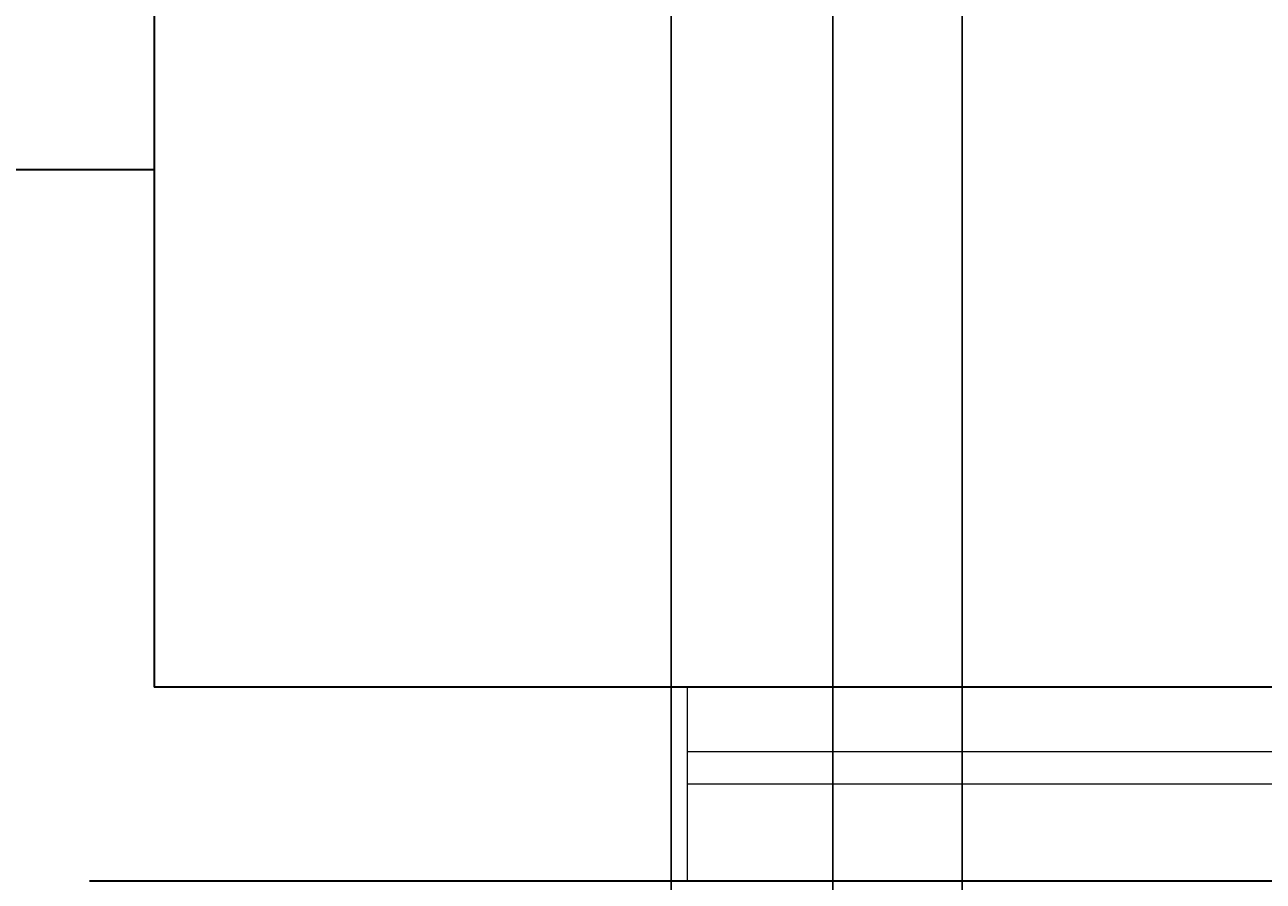
# Model space of a CAD drawing. Units: feet. Extents: x 105 to 1094, y -88 to 588.
# Tile 30 of 59: x 346 to 384, y 491 to 518. Entities that reach past the tile are written whole.
import ezdxf

# ---------------------------------------------------------------- set-up
doc = ezdxf.new("R2010")
doc.units = ezdxf.units.FT
doc.header["$MEASUREMENT"] = 0
for name, color, linetype, lineweight in [('A-ANNO-DIMS', 2, 'Continuous', 18), ('A-GLAZ', 4, 'Continuous', 18), ('A-WALL', 7, 'Continuous', 35)]:
    doc.layers.add(name, color=color, linetype=linetype, lineweight=lineweight)
doc.styles.get("Standard").update_dxf_attribs({"font": 'arial.ttf'})
doc.dimstyles.get("Standard").update_dxf_attribs({"dimtxt": 0.18, "dimasz": 0.18, "dimexe": 0.18, "dimexo": 0.0625, "dimgap": 0.09, "dimtad": 0, "dimtih": 1, "dimtoh": 1, "dimdec": 4, "dimzin": 0, "dimdsep": 46, "dimtxsty": 'Standard', "dimcen": 0.09, "dimadec": 0, "dimazin": 0, "dimtfac": 1, "dimtdec": 4, "dimtofl": 0, "dimtmove": 0, "dimatfit": 3, "dimfxl": 1, "dimtolj": 1, "dimtzin": 0, "dimarcsym": 0})

# ---------------------------------------------------------------- blocks, each defined once
blk = doc.blocks.new('WIN-TWO-LIGHT')
for p, q in [((48, 0), (48, 6)), ((24, 4), (48, 4)), ((0, 3), (48, 3))]:
    blk.add_line(p, q)
blk = doc.blocks.new('*D21')
at = {"layer": 'A-ANNO-DIMS', "color": 0, "lineweight": -2, "transparency": 16777216}
for p, q in [((849.626, 543.081), (105.458, 543.081)), ((105.638, 542.901), (105.638, 250.263)), ((105.638, -42.739), (105.638, 249.899)), ((849.626, -42.919), (105.458, -42.919))]:
    blk.add_line(p, q, dxfattribs=at)
at = {"layer": 'A-ANNO-DIMS', "color": 0, "transparency": 16777216}
for points in [[(105.608, 542.901), (105.668, 542.901), (105.638, 543.081)], [(105.608, -42.739), (105.668, -42.739), (105.638, -42.919)]]:
    blk.add_solid(points, dxfattribs=at)
at = {"layer": 'Defpoints', "color": 0, "transparency": 16777216}
for p in [(105.638, 543.081), (849.688, 543.081), (849.688, -42.919)]:
    blk.add_point(p, dxfattribs=at)
at = {"layer": 'A-ANNO-DIMS', "color": 0, "transparency": 16777216, "insert": (105.638, 250.081), "char_height": 0.18, "attachment_point": 5}
blk.add_mtext('\\A1;586', dxfattribs=at)
blk = doc.blocks.new('*D39')
at = {"layer": 'A-ANNO-DIMS', "color": 0, "lineweight": -2, "transparency": 16777216}
for p, q in [((294.688, 204.144), (294.688, 588.311)), ((294.868, 588.131), (332.47, 588.131)), ((370.508, 588.131), (332.906, 588.131)), ((370.688, 204.144), (370.688, 588.311))]:
    blk.add_line(p, q, dxfattribs=at)
at = {"layer": 'A-ANNO-DIMS', "color": 0, "transparency": 16777216}
for points in [[(294.868, 588.161), (294.868, 588.101), (294.688, 588.131)], [(370.508, 588.161), (370.508, 588.101), (370.688, 588.131)]]:
    blk.add_solid(points, dxfattribs=at)
at = {"layer": 'Defpoints', "color": 0, "transparency": 16777216}
for p in [(370.688, 588.131), (294.688, 204.081), (370.688, 204.081)]:
    blk.add_point(p, dxfattribs=at)
at = {"layer": 'A-ANNO-DIMS', "color": 0, "transparency": 16777216, "insert": (332.688, 588.131), "char_height": 0.18, "attachment_point": 5}
blk.add_mtext('\\A1;76', dxfattribs=at)
blk = doc.blocks.new('*D53')
at = {"layer": 'A-ANNO-DIMS', "color": 0, "lineweight": -2, "transparency": 16777216}
for p, q in [((365.688, 394.144), (365.688, 588.311)), ((365.868, 588.131), (389.966, 588.131)), ((414.508, 588.131), (390.411, 588.131)), ((414.688, 394.144), (414.688, 588.311))]:
    blk.add_line(p, q, dxfattribs=at)
at = {"layer": 'A-ANNO-DIMS', "color": 0, "transparency": 16777216}
for points in [[(365.868, 588.161), (365.868, 588.101), (365.688, 588.131)], [(414.508, 588.161), (414.508, 588.101), (414.688, 588.131)]]:
    blk.add_solid(points, dxfattribs=at)
at = {"layer": 'Defpoints', "color": 0, "transparency": 16777216}
for p in [(365.688, 588.131), (365.688, 394.081), (414.688, 394.081)]:
    blk.add_point(p, dxfattribs=at)
at = {"layer": 'A-ANNO-DIMS', "color": 0, "transparency": 16777216, "insert": (390.188, 588.131), "char_height": 0.18, "attachment_point": 5}
blk.add_mtext('\\A1;49', dxfattribs=at)
blk = doc.blocks.new('*D56')
at = {"layer": 'A-ANNO-DIMS', "color": 0, "lineweight": -2, "transparency": 16777216}
for p, q in [((374.688, 252.144), (374.688, 588.311)), ((374.868, 588.131), (398.466, 588.131)), ((422.508, 588.131), (398.911, 588.131)), ((422.688, 252.144), (422.688, 588.311))]:
    blk.add_line(p, q, dxfattribs=at)
at = {"layer": 'A-ANNO-DIMS', "color": 0, "transparency": 16777216}
for points in [[(374.868, 588.161), (374.868, 588.101), (374.688, 588.131)], [(422.508, 588.161), (422.508, 588.101), (422.688, 588.131)]]:
    blk.add_solid(points, dxfattribs=at)
at = {"layer": 'Defpoints', "color": 0, "transparency": 16777216}
for p in [(422.688, 588.131), (374.688, 252.081), (422.688, 252.081)]:
    blk.add_point(p, dxfattribs=at)
at = {"layer": 'A-ANNO-DIMS', "color": 0, "transparency": 16777216, "insert": (398.688, 588.131), "char_height": 0.18, "attachment_point": 5}
blk.add_mtext('\\A1;48', dxfattribs=at)

msp = doc.modelspace()

# ---------------------------------------------------------------- linework, layer by layer
at = {"layer": 'A-WALL'}
for p, q in [((349.6883, 543.0812), (349.6883, 497.0812)), ((349.6883, 513.0812), (231.6883, 513.0812)), ((438.6883, 497.0812), (349.6883, 497.0812)), ((432.6883, 491.0812), (347.6883, 491.0812))]:
    msp.add_line(p, q, dxfattribs=at)

# ---------------------------------------------------------------- block references
at = {"layer": 'A-GLAZ', "extrusion": (0, 0, -1), "zscale": -1}
msp.add_blockref('WIN-TWO-LIGHT', (-414.1886, 491.081), dxfattribs=at)

# ---------------------------------------------------------------- dimensions: what is measured, and where the dimension line sits
at = {"layer": 'A-ANNO-DIMS'}
for base, p1, p2, picture, middle in [((370.6883, 588.1312), (294.6883, 204.0812), (370.6883, 204.0812), '*D39', (332.6883, 588.1312)), ((365.6883, 588.1312), (414.6883, 394.0812), (365.6883, 394.0812), '*D53', (390.1883, 588.1312)), ((422.6883, 588.1312), (374.6883, 252.0812), (422.6883, 252.0812), '*D56', (398.6883, 588.1312))]:
    dim = msp.add_linear_dim(base=base, p1=p1, p2=p2, dimstyle='Standard', override={"dimdec": 0, "dimlfac": 1, "dimrnd": 0, "dimzin": 0, "dimdsep": 46, "dimlunit": 2}, dxfattribs=at)
    dim.commit()
    dim.dimension.update_dxf_attribs({"geometry": picture, "text_midpoint": middle})
dim = msp.add_linear_dim(base=(105.6383, 543.0812), p1=(849.6883, -42.9188), p2=(849.6883, 543.0812), angle=90, dimstyle='Standard', override={"dimdec": 0, "dimlfac": 1, "dimrnd": 0, "dimzin": 0, "dimdsep": 46, "dimlunit": 2}, dxfattribs=at)
dim.commit()
dim.dimension.update_dxf_attribs({"geometry": '*D21', "text_midpoint": (105.6383, 250.0812)})

doc.saveas('drawing.dxf')
